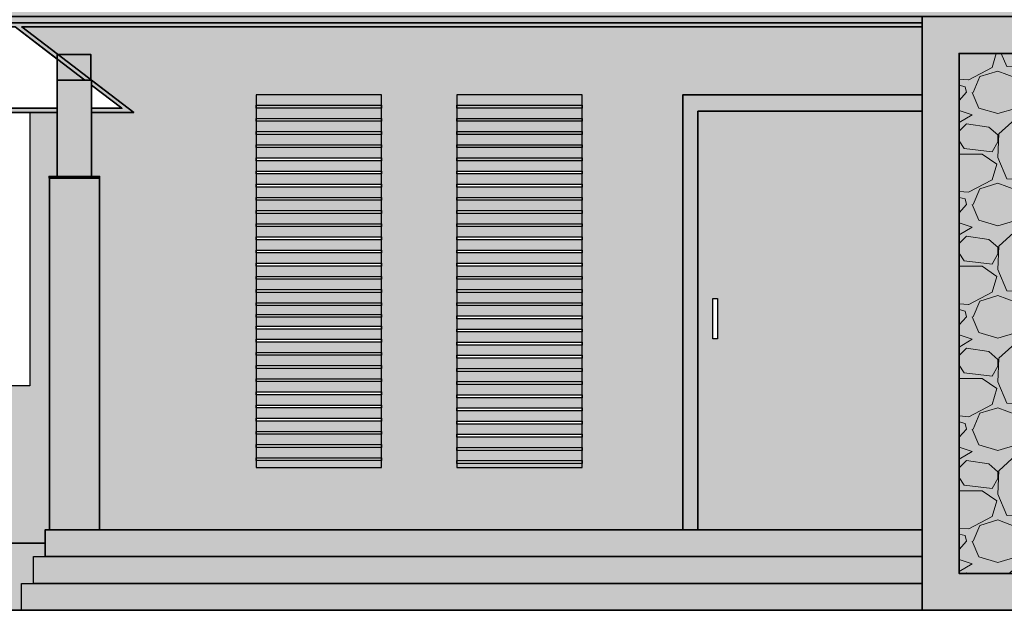
# Model space of a CAD drawing. Units: feet. Extents: x 2613 to 3913, y 950 to 1393.
# Tile 2 of 6: x 2725 to 2948, y 950 to 1083. Entities that reach past the tile are written whole.
import ezdxf

# ---------------------------------------------------------------- set-up
doc = ezdxf.new("R2010")
doc.units = ezdxf.units.FT
for name, color, linetype, lineweight in [('A-DOOR', 3, 'Continuous', 25), ('A-ELEV', 7, 'Continuous', 35), ('A-ELEV-PATT', 9, 'Continuous', 13), ('A-FLOR-STRS', 7, 'Continuous', 25), ('A-GLAZ', 4, 'Continuous', 25)]:
    doc.layers.add(name, color=color, linetype=linetype, lineweight=lineweight)

# ---------------------------------------------------------------- blocks, each defined once
blk = doc.blocks.new('WIN-LOUVRE-SHUTTER-L')
for points in [[(3513.53, 1066.37), (3485.15, 1066.37), (3485.15, 982.04), (3513.53, 982.04)], [(3485.15, 1064.05), (3513.53, 1064.05), (3513.53, 1063.39), (3485.15, 1063.39)], [(3485.15, 1061.07), (3513.53, 1061.07), (3513.53, 1060.41), (3485.15, 1060.41)], [(3485.15, 1058.09), (3513.53, 1058.09), (3513.53, 1057.43), (3485.15, 1057.43)], [(3485.15, 1055.11), (3513.53, 1055.11), (3513.53, 1054.45), (3485.15, 1054.45)], [(3485.15, 1052.13), (3513.53, 1052.13), (3513.53, 1051.47), (3485.15, 1051.47)], [(3485.15, 1049.15), (3513.53, 1049.15), (3513.53, 1048.49), (3485.15, 1048.49)], [(3485.15, 1046.18), (3513.53, 1046.18), (3513.53, 1045.51), (3485.15, 1045.51)], [(3485.15, 1043.2), (3513.53, 1043.2), (3513.53, 1042.53), (3485.15, 1042.53)], [(3485.15, 1040.22), (3513.53, 1040.22), (3513.53, 1039.56), (3485.15, 1039.56)], [(3485.15, 1037.24), (3513.53, 1037.24), (3513.53, 1036.58), (3485.15, 1036.58)], [(3485.15, 1034.26), (3513.53, 1034.26), (3513.53, 1033.6), (3485.15, 1033.6)], [(3485.15, 1031.28), (3513.53, 1031.28), (3513.53, 1030.62), (3485.15, 1030.62)], [(3485.15, 1028.3), (3513.53, 1028.3), (3513.53, 1027.64), (3485.15, 1027.64)], [(3485.15, 1025.32), (3513.53, 1025.32), (3513.53, 1024.66), (3485.15, 1024.66)], [(3485.15, 1022.34), (3513.53, 1022.34), (3513.53, 1021.68), (3485.15, 1021.68)], [(3485.15, 1019.36), (3513.53, 1019.36), (3513.53, 1018.7), (3485.15, 1018.7)], [(3485.15, 1016.71), (3513.53, 1016.71), (3513.53, 1016.05), (3485.15, 1016.05)], [(3485.15, 1014.07), (3513.53, 1014.07), (3513.53, 1013.4), (3485.15, 1013.4)], [(3485.15, 1011.09), (3513.53, 1011.09), (3513.53, 1010.43), (3485.15, 1010.43)], [(3485.15, 1008.11), (3513.53, 1008.11), (3513.53, 1007.45), (3485.15, 1007.45)], [(3485.15, 1005.13), (3513.53, 1005.13), (3513.53, 1004.47), (3485.15, 1004.47)], [(3485.15, 1002.15), (3513.53, 1002.15), (3513.53, 1001.49), (3485.15, 1001.49)], [(3485.15, 999.17), (3513.53, 999.17), (3513.53, 998.51), (3485.15, 998.51)], [(3485.15, 996.19), (3513.53, 996.19), (3513.53, 995.53), (3485.15, 995.53)], [(3485.15, 993.21), (3513.53, 993.21), (3513.53, 992.55), (3485.15, 992.55)], [(3485.15, 990.23), (3513.53, 990.23), (3513.53, 989.57), (3485.15, 989.57)], [(3485.15, 987.25), (3513.53, 987.25), (3513.53, 986.59), (3485.15, 986.59)], [(3485.15, 984.27), (3513.53, 984.27), (3513.53, 983.61), (3485.15, 983.61)]]:
    blk.add_lwpolyline(points, close=True)
blk = doc.blocks.new('WIN-LOUVRE-SHUTTER-R')
for points in [[(3559, 1066.37), (3530.62, 1066.37), (3530.62, 982.04), (3559, 982.04)], [(3530.62, 1064.05), (3559, 1064.05), (3559, 1063.39), (3530.62, 1063.39)], [(3530.62, 1061.07), (3559, 1061.07), (3559, 1060.41), (3530.62, 1060.41)], [(3530.62, 1058.09), (3559, 1058.09), (3559, 1057.43), (3530.62, 1057.43)], [(3530.62, 1055.11), (3559, 1055.11), (3559, 1054.45), (3530.62, 1054.45)], [(3530.62, 1052.13), (3559, 1052.13), (3559, 1051.47), (3530.62, 1051.47)], [(3530.62, 1049.15), (3559, 1049.15), (3559, 1048.49), (3530.62, 1048.49)], [(3530.62, 1046.18), (3559, 1046.18), (3559, 1045.51), (3530.62, 1045.51)], [(3530.62, 1043.2), (3559, 1043.2), (3559, 1042.53), (3530.62, 1042.53)], [(3530.62, 1040.22), (3559, 1040.22), (3559, 1039.56), (3530.62, 1039.56)], [(3530.62, 1037.24), (3559, 1037.24), (3559, 1036.58), (3530.62, 1036.58)], [(3530.62, 1034.26), (3559, 1034.26), (3559, 1033.6), (3530.62, 1033.6)], [(3530.62, 1031.28), (3559, 1031.28), (3559, 1030.62), (3530.62, 1030.62)], [(3530.62, 1028.3), (3559, 1028.3), (3559, 1027.64), (3530.62, 1027.64)], [(3530.62, 1025.32), (3559, 1025.32), (3559, 1024.66), (3530.62, 1024.66)], [(3530.62, 1022.34), (3559, 1022.34), (3559, 1021.68), (3530.62, 1021.68)], [(3530.62, 1019.36), (3559, 1019.36), (3559, 1018.7), (3530.62, 1018.7)], [(3530.62, 1016.38), (3559, 1016.38), (3559, 1015.72), (3530.62, 1015.72)], [(3530.62, 1013.4), (3559, 1013.4), (3559, 1012.74), (3530.62, 1012.74)], [(3530.62, 1010.43), (3559, 1010.43), (3559, 1009.76), (3530.62, 1009.76)], [(3530.62, 1007.45), (3559, 1007.45), (3559, 1006.78), (3530.62, 1006.78)], [(3530.62, 1004.47), (3559, 1004.47), (3559, 1003.81), (3530.62, 1003.81)], [(3530.62, 1001.49), (3559, 1001.49), (3559, 1000.83), (3530.62, 1000.83)], [(3530.62, 998.51), (3559, 998.51), (3559, 997.85), (3530.62, 997.85)], [(3530.62, 995.53), (3559, 995.53), (3559, 994.87), (3530.62, 994.87)], [(3530.62, 992.55), (3559, 992.55), (3559, 991.89), (3530.62, 991.89)], [(3530.62, 989.57), (3559, 989.57), (3559, 988.91), (3530.62, 988.91)], [(3530.62, 986.59), (3559, 986.59), (3559, 985.93), (3530.62, 985.93)], [(3530.62, 983.61), (3559, 983.61), (3559, 982.95), (3530.62, 982.95)]]:
    blk.add_lwpolyline(points, close=True)

msp = doc.modelspace()

# ---------------------------------------------------------------- hatches: boundary and pattern name
at = {"layer": 'A-ELEV-PATT'}
h = msp.add_hatch(color=256, dxfattribs=at)
h.dxf.hatch_style = 1
h.paths.add_polyline_path([(3108.91, 1328.81), (3061.44, 1376.28), (2929.45, 1244.29), (2929.45, 1223.38), (2942.09, 1223.38), (2942.09, 1215.5), (2929.45, 1215.5), (2929.45, 1084.12), (3108.91, 1084.12), (3108.91, 1199.69), (3106.87, 1199.69), (3106.87, 1128.72), (3017.91, 1128.72), (3017.91, 1199.69), (3008.08, 1199.69), (3008.08, 1180.01), (3007.65, 1180.01), (3007.65, 1199.69), (3004.75, 1199.69), (3004.75, 1206.47), (3108.91, 1206.47)])
h.paths.add_polyline_path([(3061.44, 1376.28), (3193.8, 1243.92), (3193.8, 1233.84), (3204.34, 1246.9), (3061.54, 1389.71), (2918.82, 1247), (2929.45, 1233.69), (2929.45, 1244.29)])
h.paths.add_polyline_path([(3061.54, 1389.71), (3204.34, 1246.9), (3206.69, 1248.02), (3061.63, 1393.09), (2916.59, 1248.06), (2918.82, 1247)])
h.paths.add_polyline_path([(2925.65, 1257.12), (2667.59, 1257.12), (2651.33, 1257.12), (2651.33, 1252.28), (2920.82, 1252.28)])
h.paths.add_polyline_path([(2920.82, 1252.28), (2651.33, 1252.28, -0.144454), (2652.15, 1251.12), (2667.59, 1251.12), (2919.65, 1251.12)])
h.paths.add_polyline_path([(2918.82, 1247), (2916.59, 1248.06), (2919.65, 1251.12), (2667.59, 1251.12), (2652.15, 1251.12), (2667.59, 1229.14), (2667.59, 1233.69), (2929.45, 1233.69)])
h.paths.add_polyline_path([(2710.6, 1223.38), (2929.45, 1223.38), (2929.45, 1233.69), (2667.59, 1233.69), (2667.59, 1229.14), (2667.59, 1201.16), (2720.67, 1201.16), (2710.6, 1215.5)])
h.paths.add_polyline_path([(2942.09, 1223.38), (2710.6, 1223.38), (2710.6, 1215.5), (2921.48, 1215.5), (2942.09, 1215.5)])
h.paths.add_polyline_path([(2929.45, 1215.5), (2921.48, 1215.5), (2710.6, 1215.5), (2733.47, 1182.94), (2733.47, 1195.74), (2741.22, 1195.74), (2929.45, 1195.74)])
h.paths.add_polyline_path([(2721, 1200.68), (2661.89, 1200.68), (2661.89, 1195.74), (2724.47, 1195.74)])
h.paths.add_polyline_path([(2733.47, 1182.94), (2727.27, 1191.76), (2727.27, 1133.88), (2731.7, 1133.88), (2731.7, 1169.74), (2731.61, 1169.74), (2731.61, 1170.13), (2733.47, 1170.13)])
h.paths.add_polyline_path([(2929.45, 1183.04), (2741.22, 1183.04), (2741.22, 1170.13), (2743.07, 1170.13), (2743.07, 1169.74), (2743.07, 1112.32), (2759.57, 1112.32), (2759.57, 1167.82), (2763.7, 1167.82), (2763.7, 1112.32), (2781.75, 1112.32), (2781.75, 1167.82), (2785.87, 1167.82), (2785.87, 1112.32), (2803.92, 1112.32), (2803.92, 1167.82), (2808.05, 1167.82), (2808.05, 1112.32), (2826.09, 1112.32), (2826.09, 1167.82), (2830.22, 1167.82), (2830.22, 1112.32), (2875.17, 1112.32), (2875.17, 1171.49), (2929.45, 1171.49)])
h.paths.add_polyline_path([(2731.7, 1133.88), (2661.89, 1133.88), (2661.89, 1084.12), (2730.99, 1084.12), (2730.99, 1112.32), (2731.7, 1112.32)])
h.paths.add_polyline_path([(2929.45, 1112.32), (2730.99, 1112.32), (2730.99, 1084.12), (2929.45, 1084.12)])
h.paths.add_polyline_path([(2929.45, 1084.12), (2730.99, 1084.12), (2661.89, 1084.12), (2612.72, 1084.12), (2612.72, 1082.68), (2929.45, 1082.68)])
h.paths.add_polyline_path([(2929.45, 1082.68), (2612.72, 1082.68), (2639.32, 1062.44), (2733.47, 1062.44), (2733.47, 1063.35), (2639.62, 1063.35), (2615.43, 1081.77), (2723.91, 1081.77), (2739.71, 1069.74), (2741.22, 1069.74), (2725.42, 1081.77), (2929.45, 1081.77)])
h.paths.add_polyline_path([(2671.42, 1081.77), (2668.07, 1081.77), (2692.27, 1063.35), (2695.62, 1063.35)], flags=17)
h.paths.add_polyline_path([(2741.22, 1069.74), (2741.22, 1068.59), (2748.11, 1063.35), (2741.22, 1063.35), (2741.22, 1062.44), (2750.82, 1062.44)], flags=17)
h.paths.add_polyline_path([(2929.45, 1081.77), (2725.42, 1081.77), (2750.82, 1062.44), (2741.22, 1062.44), (2741.22, 1047.95), (2743.07, 1047.95), (2743.07, 1047.56), (2743.07, 967.97), (2875.17, 967.97), (2875.17, 1066.37), (2929.45, 1066.37)])
h.paths.add_polyline_path([(2778.55, 1066.37), (2806.94, 1066.37), (2806.94, 982.04), (2778.55, 982.04)], flags=16)
h.paths.add_polyline_path([(2778.55, 1064.05), (2806.94, 1064.05), (2806.94, 1063.39), (2778.55, 1063.39)], flags=16)
h.paths.add_polyline_path([(2778.55, 1061.07), (2806.94, 1061.07), (2806.94, 1060.41), (2778.55, 1060.41)], flags=0)
h.paths.add_polyline_path([(2778.55, 1058.09), (2806.94, 1058.09), (2806.94, 1057.43), (2778.55, 1057.43)], flags=0)
h.paths.add_polyline_path([(2778.55, 1055.11), (2806.94, 1055.11), (2806.94, 1054.45), (2778.55, 1054.45)], flags=0)
h.paths.add_polyline_path([(2778.55, 1052.13), (2806.94, 1052.13), (2806.94, 1051.47), (2778.55, 1051.47)], flags=0)
h.paths.add_polyline_path([(2778.55, 1049.15), (2806.94, 1049.15), (2806.94, 1048.49), (2778.55, 1048.49)], flags=0)
h.paths.add_polyline_path([(2778.55, 1046.18), (2806.94, 1046.18), (2806.94, 1045.51), (2778.55, 1045.51)], flags=0)
h.paths.add_polyline_path([(2778.55, 1043.2), (2806.94, 1043.2), (2806.94, 1042.53), (2778.55, 1042.53)], flags=0)
h.paths.add_polyline_path([(2778.55, 1040.22), (2806.94, 1040.22), (2806.94, 1039.56), (2778.55, 1039.56)], flags=0)
h.paths.add_polyline_path([(2778.55, 1037.24), (2806.94, 1037.24), (2806.94, 1036.58), (2778.55, 1036.58)], flags=0)
h.paths.add_polyline_path([(2778.55, 1034.26), (2806.94, 1034.26), (2806.94, 1033.6), (2778.55, 1033.6)], flags=0)
h.paths.add_polyline_path([(2778.55, 1031.28), (2806.94, 1031.28), (2806.94, 1030.62), (2778.55, 1030.62)], flags=0)
h.paths.add_polyline_path([(2778.55, 1028.3), (2806.94, 1028.3), (2806.94, 1027.64), (2778.55, 1027.64)], flags=0)
h.paths.add_polyline_path([(2778.55, 1025.32), (2806.94, 1025.32), (2806.94, 1024.66), (2778.55, 1024.66)], flags=0)
h.paths.add_polyline_path([(2778.55, 1022.34), (2806.94, 1022.34), (2806.94, 1021.68), (2778.55, 1021.68)], flags=0)
h.paths.add_polyline_path([(2778.55, 1019.36), (2806.94, 1019.36), (2806.94, 1018.7), (2778.55, 1018.7)], flags=0)
h.paths.add_polyline_path([(2778.55, 1016.71), (2806.94, 1016.71), (2806.94, 1016.05), (2778.55, 1016.05)], flags=0)
h.paths.add_polyline_path([(2824.02, 1066.37), (2852.41, 1066.37), (2852.41, 982.04), (2824.02, 982.04)], flags=16)
h.paths.add_polyline_path([(2778.55, 1014.07), (2806.94, 1014.07), (2806.94, 1013.4), (2778.55, 1013.4)], flags=0)
h.paths.add_polyline_path([(2824.02, 1064.05), (2852.41, 1064.05), (2852.41, 1063.39), (2824.02, 1063.39)], flags=16)
h.paths.add_polyline_path([(2824.02, 1061.07), (2852.41, 1061.07), (2852.41, 1060.41), (2824.02, 1060.41)], flags=0)
h.paths.add_polyline_path([(2824.02, 1058.09), (2852.41, 1058.09), (2852.41, 1057.43), (2824.02, 1057.43)], flags=0)
h.paths.add_polyline_path([(2824.02, 1055.11), (2852.41, 1055.11), (2852.41, 1054.45), (2824.02, 1054.45)], flags=16)
h.paths.add_polyline_path([(2824.02, 1052.13), (2852.41, 1052.13), (2852.41, 1051.47), (2824.02, 1051.47)], flags=0)
h.paths.add_polyline_path([(2778.55, 1011.09), (2806.94, 1011.09), (2806.94, 1010.43), (2778.55, 1010.43)], flags=0)
h.paths.add_polyline_path([(2824.02, 1049.15), (2852.41, 1049.15), (2852.41, 1048.49), (2824.02, 1048.49)], flags=0)
h.paths.add_polyline_path([(2824.02, 1046.18), (2852.41, 1046.18), (2852.41, 1045.51), (2824.02, 1045.51)], flags=0)
h.paths.add_polyline_path([(2824.02, 1043.2), (2852.41, 1043.2), (2852.41, 1042.53), (2824.02, 1042.53)], flags=0)
h.paths.add_polyline_path([(2778.55, 1008.11), (2806.94, 1008.11), (2806.94, 1007.45), (2778.55, 1007.45)], flags=0)
h.paths.add_polyline_path([(2824.02, 1040.22), (2852.41, 1040.22), (2852.41, 1039.56), (2824.02, 1039.56)], flags=0)
h.paths.add_polyline_path([(2824.02, 1037.24), (2852.41, 1037.24), (2852.41, 1036.58), (2824.02, 1036.58)], flags=0)
h.paths.add_polyline_path([(2778.55, 1005.13), (2806.94, 1005.13), (2806.94, 1004.47), (2778.55, 1004.47)], flags=0)
h.paths.add_polyline_path([(2824.02, 1034.26), (2852.41, 1034.26), (2852.41, 1033.6), (2824.02, 1033.6)], flags=0)
h.paths.add_polyline_path([(2824.02, 1031.28), (2852.41, 1031.28), (2852.41, 1030.62), (2824.02, 1030.62)], flags=0)
h.paths.add_polyline_path([(2778.55, 1002.15), (2806.94, 1002.15), (2806.94, 1001.49), (2778.55, 1001.49)], flags=0)
h.paths.add_polyline_path([(2824.02, 1028.3), (2852.41, 1028.3), (2852.41, 1027.64), (2824.02, 1027.64)], flags=0)
h.paths.add_polyline_path([(2778.55, 999.17), (2806.94, 999.17), (2806.94, 998.51), (2778.55, 998.51)], flags=0)
h.paths.add_polyline_path([(2824.02, 1025.32), (2852.41, 1025.32), (2852.41, 1024.66), (2824.02, 1024.66)], flags=0)
h.paths.add_polyline_path([(2824.02, 1022.34), (2852.41, 1022.34), (2852.41, 1021.68), (2824.02, 1021.68)], flags=0)
h.paths.add_polyline_path([(2778.55, 996.19), (2806.94, 996.19), (2806.94, 995.53), (2778.55, 995.53)], flags=0)
h.paths.add_polyline_path([(2824.02, 1019.36), (2852.41, 1019.36), (2852.41, 1018.7), (2824.02, 1018.7)], flags=0)
h.paths.add_polyline_path([(2778.55, 993.21), (2806.94, 993.21), (2806.94, 992.55), (2778.55, 992.55)], flags=0)
h.paths.add_polyline_path([(2824.02, 1016.38), (2852.41, 1016.38), (2852.41, 1015.72), (2824.02, 1015.72)], flags=0)
h.paths.add_polyline_path([(2824.02, 1013.4), (2852.41, 1013.4), (2852.41, 1012.74), (2824.02, 1012.74)], flags=0)
h.paths.add_polyline_path([(2778.55, 990.23), (2806.94, 990.23), (2806.94, 989.57), (2778.55, 989.57)], flags=0)
h.paths.add_polyline_path([(2824.02, 1010.43), (2852.41, 1010.43), (2852.41, 1009.76), (2824.02, 1009.76)], flags=0)
h.paths.add_polyline_path([(2778.55, 987.25), (2806.94, 987.25), (2806.94, 986.59), (2778.55, 986.59)], flags=0)
h.paths.add_polyline_path([(2824.02, 1007.45), (2852.41, 1007.45), (2852.41, 1006.78), (2824.02, 1006.78)], flags=0)
h.paths.add_polyline_path([(2778.55, 984.27), (2806.94, 984.27), (2806.94, 983.61), (2778.55, 983.61)], flags=0)
h.paths.add_polyline_path([(2824.02, 1004.47), (2852.41, 1004.47), (2852.41, 1003.81), (2824.02, 1003.81)], flags=0)
h.paths.add_polyline_path([(2824.02, 1001.49), (2852.41, 1001.49), (2852.41, 1000.83), (2824.02, 1000.83)], flags=0)
h.paths.add_polyline_path([(2824.02, 998.51), (2852.41, 998.51), (2852.41, 997.85), (2824.02, 997.85)], flags=0)
h.paths.add_polyline_path([(2824.02, 995.53), (2852.41, 995.53), (2852.41, 994.87), (2824.02, 994.87)], flags=0)
h.paths.add_polyline_path([(2824.02, 992.55), (2852.41, 992.55), (2852.41, 991.89), (2824.02, 991.89)], flags=0)
h.paths.add_polyline_path([(2824.02, 989.57), (2852.41, 989.57), (2852.41, 988.91), (2824.02, 988.91)], flags=0)
h.paths.add_polyline_path([(2824.02, 986.59), (2852.41, 986.59), (2852.41, 985.93), (2824.02, 985.93)], flags=0)
h.paths.add_polyline_path([(2824.02, 983.61), (2852.41, 983.61), (2852.41, 982.95), (2824.02, 982.95)], flags=0)
h.paths.add_polyline_path([(2731.7, 1047.56), (2731.61, 1047.56), (2731.61, 1047.95), (2733.47, 1047.95), (2733.47, 1062.44), (2727.27, 1062.44), (2727.27, 1000.58), (2667.59, 1000.58), (2667.59, 1062.44), (2664.87, 1062.44), (2664.87, 965.01), (2730.76, 964.93), (2730.76, 967.97), (2731.7, 967.97)])
h.paths.add_polyline_path([(2728.06, 961.9), (2730.76, 961.9), (2730.76, 964.93), (2663.94, 964.93), (2663.94, 949.74), (2725.36, 949.74), (2725.36, 955.82), (2728.06, 955.82)])
h.paths.add_polyline_path([(2929.45, 967.97), (2730.76, 967.97), (2730.76, 961.9), (2929.45, 961.9)])
h.paths.add_polyline_path([(2929.45, 961.9), (2730.76, 961.9), (2728.06, 961.9), (2728.06, 955.82), (2929.45, 955.82)])
h.paths.add_polyline_path([(2929.45, 955.82), (2728.06, 955.82), (2725.36, 955.82), (2725.36, 949.74), (2929.45, 949.74)])
h.paths.add_polyline_path([(2741.22, 1069.74), (2733.47, 1069.74), (2733.47, 1047.95), (2741.22, 1047.95)], flags=17)
h.paths.add_polyline_path([(2741.22, 1195.74), (2733.47, 1195.74), (2733.47, 1182.94), (2733.47, 1170.13), (2741.22, 1170.13), (2741.22, 1183.04)])
h.paths.add_polyline_path([(3193.8, 1084.12), (2929.45, 1084.12), (2929.45, 1082.68), (2929.45, 1081.77), (2929.45, 1066.37), (2929.45, 949.74), (3193.8, 949.74)])
h.paths.add_polyline_path([(2937.79, 1075.78), (3185.46, 1075.78), (3185.46, 958.09), (2937.79, 958.09)], flags=16)
h.paths.add_polyline_path([(3011.76, 1075.78), (3104.46, 1075.78), (3104.46, 993.6), (3011.76, 993.6)], flags=0)
h.paths.add_polyline_path([(3015.24, 1075.78), (3016.57, 1075.78), (3016.57, 1060.85), (3043.1, 1060.85), (3043.1, 1075.78), (3045.77, 1075.78), (3045.77, 997.08), (3070.45, 997.08), (3070.45, 1075.78), (3073.12, 1075.78), (3073.12, 1060.85), (3099.64, 1060.85), (3099.64, 1075.78), (3100.98, 1075.78), (3100.98, 997.08), (3099.64, 997.08), (3015.24, 997.08)], flags=0)
h = msp.add_hatch(color=256, dxfattribs=at)
h.dxf.hatch_style = 1
h.paths.add_polyline_path([(2768.1, 1195.09), (2741.95, 1195.09), (2741.95, 1183.7), (2768.1, 1183.7)])
h.paths.add_polyline_path([(2794.91, 1195.09), (2768.76, 1195.09), (2768.76, 1183.7), (2794.91, 1183.7)])
h.paths.add_polyline_path([(2821.72, 1195.09), (2795.57, 1195.09), (2795.57, 1183.7), (2821.72, 1183.7)])
h.paths.add_polyline_path([(2848.53, 1195.09), (2822.38, 1195.09), (2822.38, 1183.7), (2848.53, 1183.7)])
h.paths.add_polyline_path([(2875.34, 1195.09), (2849.19, 1195.09), (2849.19, 1183.7), (2875.34, 1183.7)])
h.paths.add_polyline_path([(2683.29, 1193.04), (2670.29, 1193.04), (2670.29, 1190.17), (2683.29, 1190.17)])
h.paths.add_polyline_path([(2696.31, 1193.04), (2683.32, 1193.04), (2683.32, 1190.17), (2696.31, 1190.17)])
h.paths.add_polyline_path([(2696.31, 1190.14), (2683.32, 1190.14), (2683.32, 1187.27), (2696.31, 1187.27)])
h.paths.add_polyline_path([(2683.29, 1190.14), (2670.29, 1190.14), (2670.29, 1187.27), (2683.29, 1187.27)])
h.paths.add_polyline_path([(2683.29, 1187.24), (2670.29, 1187.24), (2670.29, 1184.37), (2683.29, 1184.37)])
h.paths.add_polyline_path([(2696.31, 1187.24), (2683.32, 1187.24), (2683.32, 1184.37), (2696.31, 1184.37)])
h.paths.add_polyline_path([(2683.29, 1184.34), (2670.29, 1184.34), (2670.29, 1181.47), (2683.29, 1181.47)])
h.paths.add_polyline_path([(2696.31, 1184.34), (2683.32, 1184.34), (2683.32, 1181.47), (2696.31, 1181.47)])
h.paths.add_polyline_path([(2683.29, 1181.44), (2670.29, 1181.44), (2670.29, 1178.57), (2683.29, 1178.57)])
h.paths.add_polyline_path([(2696.31, 1181.44), (2683.32, 1181.44), (2683.32, 1178.57), (2696.31, 1178.57)])
h.paths.add_polyline_path([(2696.31, 1178.53), (2683.32, 1178.53), (2683.32, 1175.67), (2696.31, 1175.67)])
h.paths.add_polyline_path([(2683.29, 1178.53), (2670.29, 1178.53), (2670.29, 1175.67), (2683.29, 1175.67)])
h.paths.add_polyline_path([(2683.29, 1175.63), (2670.29, 1175.63), (2670.29, 1172.76), (2683.29, 1172.76)])
h.paths.add_polyline_path([(2696.31, 1175.63), (2683.32, 1175.63), (2683.32, 1172.76), (2696.31, 1172.76)])
h.paths.add_polyline_path([(2683.29, 1172.73), (2670.29, 1172.73), (2670.29, 1169.86), (2683.29, 1169.86)])
h.paths.add_polyline_path([(2696.31, 1172.73), (2683.32, 1172.73), (2683.32, 1169.86), (2696.31, 1169.86)])
h.paths.add_polyline_path([(2696.31, 1169.83), (2683.32, 1169.83), (2683.32, 1166.96), (2696.31, 1166.96)])
h.paths.add_polyline_path([(2683.29, 1169.83), (2670.29, 1169.83), (2670.29, 1166.96), (2683.29, 1166.96)])
h.paths.add_polyline_path([(2696.31, 1166.93), (2683.32, 1166.93), (2683.32, 1164.06), (2696.31, 1164.06)])
h.paths.add_polyline_path([(2683.29, 1166.93), (2670.29, 1166.93), (2670.29, 1164.06), (2683.29, 1164.06)])
h.paths.add_polyline_path([(2683.29, 1164.03), (2670.29, 1164.03), (2670.29, 1161.16), (2683.29, 1161.16)])
h.paths.add_polyline_path([(2696.31, 1164.03), (2683.32, 1164.03), (2683.32, 1161.16), (2696.31, 1161.16)])
h.paths.add_polyline_path([(2696.31, 1161.12), (2683.32, 1161.12), (2683.32, 1158.25), (2696.31, 1158.25)])
h.paths.add_polyline_path([(2683.29, 1161.12), (2670.29, 1161.12), (2670.29, 1158.25), (2683.29, 1158.25)])
h.paths.add_polyline_path([(2683.29, 1158.22), (2670.29, 1158.22), (2670.29, 1155.35), (2683.29, 1155.35)])
h.paths.add_polyline_path([(2696.31, 1158.22), (2683.32, 1158.22), (2683.32, 1155.35), (2696.31, 1155.35)])
h.paths.add_polyline_path([(2696.31, 1155.32), (2683.32, 1155.32), (2683.32, 1152.45), (2696.31, 1152.45)])
h.paths.add_polyline_path([(2683.29, 1155.32), (2670.29, 1155.32), (2670.29, 1152.45), (2683.29, 1152.45)])
h.paths.add_polyline_path([(2683.29, 1152.42), (2670.29, 1152.42), (2670.29, 1149.55), (2683.29, 1149.55)])
h.paths.add_polyline_path([(2696.31, 1152.42), (2683.32, 1152.42), (2683.32, 1149.55), (2696.31, 1149.55)])
h.paths.add_polyline_path([(2683.29, 1149.52), (2670.29, 1149.52), (2670.29, 1146.65), (2683.29, 1146.65)])
h.paths.add_polyline_path([(2696.31, 1149.52), (2683.32, 1149.52), (2683.32, 1146.65), (2696.31, 1146.65)])
h.paths.add_polyline_path([(2696.31, 1146.61), (2683.32, 1146.61), (2683.32, 1143.75), (2696.31, 1143.75)])
h.paths.add_polyline_path([(2683.29, 1146.61), (2670.29, 1146.61), (2670.29, 1143.75), (2683.29, 1143.75)])
h.paths.add_polyline_path([(2683.29, 1143.71), (2670.29, 1143.71), (2670.29, 1140.84), (2683.29, 1140.84)])
h.paths.add_polyline_path([(2696.31, 1143.71), (2683.32, 1143.71), (2683.32, 1140.84), (2696.31, 1140.84)])
h.paths.add_polyline_path([(2683.29, 1140.81), (2670.29, 1140.81), (2670.29, 1137.94), (2683.29, 1137.94)])
h.paths.add_polyline_path([(2696.31, 1140.81), (2683.32, 1140.81), (2683.32, 1137.94), (2696.31, 1137.94)])
h.paths.add_polyline_path([(2683.29, 1137.91), (2670.29, 1137.91), (2670.29, 1136.58), (2683.29, 1136.58)])
h.paths.add_polyline_path([(2696.31, 1137.91), (2683.32, 1137.91), (2683.32, 1136.58), (2696.31, 1136.58)])
h.paths.add_polyline_path([(3074.7, 1198.4), (3050.02, 1198.4), (3050.02, 1130.01), (3074.7, 1130.01)])
h.paths.add_polyline_path([(3047.34, 1198.4), (3019.29, 1198.4), (3019.29, 1184.76), (3047.34, 1184.76)])
h.paths.add_polyline_path([(3047.34, 1183.78), (3019.29, 1183.78), (3019.29, 1130.01), (3047.34, 1130.01)])
h.paths.add_polyline_path([(3105.48, 1198.4), (3077.37, 1198.4), (3077.37, 1184.76), (3105.48, 1184.76)])
h.paths.add_polyline_path([(3105.48, 1183.78), (3077.37, 1183.78), (3077.37, 1130.01), (3105.48, 1130.01)])
h.paths.add_polyline_path([(3070.45, 1075.78), (3045.77, 1075.78), (3045.77, 997.08), (3070.45, 997.08)])
h.paths.add_polyline_path([(3099.64, 1075.78), (3073.12, 1075.78), (3073.12, 1060.85), (3099.64, 1060.85)])
h.paths.add_polyline_path([(3099.64, 1059.87), (3073.12, 1059.87), (3073.12, 997.08), (3099.64, 997.08)])
h.paths.add_polyline_path([(3043.1, 1075.78), (3016.57, 1075.78), (3016.57, 1060.85), (3043.1, 1060.85)])
h.paths.add_polyline_path([(3043.1, 1059.87), (3016.57, 1059.87), (3016.57, 997.08), (3043.1, 997.08)])
h.paths.add_polyline_path([(2683.29, 1059.73), (2670.29, 1059.73), (2670.29, 1056.87), (2683.29, 1056.87)])
h.paths.add_polyline_path([(2696.31, 1059.73), (2683.32, 1059.73), (2683.32, 1056.87), (2696.31, 1056.87)])
h.paths.add_polyline_path([(2696.31, 1056.83), (2683.32, 1056.83), (2683.32, 1053.96), (2696.31, 1053.96)])
h.paths.add_polyline_path([(2683.29, 1056.83), (2670.29, 1056.83), (2670.29, 1053.96), (2683.29, 1053.96)])
h.paths.add_polyline_path([(2683.29, 1053.93), (2670.29, 1053.93), (2670.29, 1051.06), (2683.29, 1051.06)])
h.paths.add_polyline_path([(2696.31, 1053.93), (2683.32, 1053.93), (2683.32, 1051.06), (2696.31, 1051.06)])
h.paths.add_polyline_path([(2683.29, 1051.03), (2670.29, 1051.03), (2670.29, 1048.16), (2683.29, 1048.16)])
h.paths.add_polyline_path([(2696.31, 1051.03), (2683.32, 1051.03), (2683.32, 1048.16), (2696.31, 1048.16)])
h.paths.add_polyline_path([(2683.29, 1048.13), (2670.29, 1048.13), (2670.29, 1045.26), (2683.29, 1045.26)])
h.paths.add_polyline_path([(2696.31, 1048.13), (2683.32, 1048.13), (2683.32, 1045.26), (2696.31, 1045.26)])
h.paths.add_polyline_path([(2696.31, 1045.23), (2683.32, 1045.23), (2683.32, 1042.36), (2696.31, 1042.36)])
h.paths.add_polyline_path([(2683.29, 1045.23), (2670.29, 1045.23), (2670.29, 1042.36), (2683.29, 1042.36)])
h.paths.add_polyline_path([(2683.29, 1042.32), (2670.29, 1042.32), (2670.29, 1039.46), (2683.29, 1039.46)])
h.paths.add_polyline_path([(2696.31, 1042.32), (2683.32, 1042.32), (2683.32, 1039.46), (2696.31, 1039.46)])
h.paths.add_polyline_path([(2696.31, 1039.42), (2683.32, 1039.42), (2683.32, 1036.55), (2696.31, 1036.55)])
h.paths.add_polyline_path([(2683.29, 1039.42), (2670.29, 1039.42), (2670.29, 1036.55), (2683.29, 1036.55)])
h.paths.add_polyline_path([(2683.29, 1036.52), (2670.29, 1036.52), (2670.29, 1033.65), (2683.29, 1033.65)])
h.paths.add_polyline_path([(2696.31, 1036.52), (2683.32, 1036.52), (2683.32, 1033.65), (2696.31, 1033.65)])
h.paths.add_polyline_path([(2696.31, 1033.62), (2683.32, 1033.62), (2683.32, 1030.75), (2696.31, 1030.75)])
h.paths.add_polyline_path([(2683.29, 1033.62), (2670.29, 1033.62), (2670.29, 1030.75), (2683.29, 1030.75)])
h.paths.add_polyline_path([(2696.31, 1030.72), (2683.32, 1030.72), (2683.32, 1027.85), (2696.31, 1027.85)])
h.paths.add_polyline_path([(2683.29, 1030.72), (2670.29, 1030.72), (2670.29, 1027.85), (2683.29, 1027.85)])
h.paths.add_polyline_path([(2683.29, 1027.82), (2670.29, 1027.82), (2670.29, 1024.95), (2683.29, 1024.95)])
h.paths.add_polyline_path([(2696.31, 1027.82), (2683.32, 1027.82), (2683.32, 1024.95), (2696.31, 1024.95)])
h.paths.add_polyline_path([(2696.31, 1024.91), (2683.32, 1024.91), (2683.32, 1022.05), (2696.31, 1022.05)])
h.paths.add_polyline_path([(2683.29, 1024.91), (2670.29, 1024.91), (2670.29, 1022.05), (2683.29, 1022.05)])
h.paths.add_polyline_path([(2683.29, 1022.01), (2670.29, 1022.01), (2670.29, 1019.14), (2683.29, 1019.14)])
h.paths.add_polyline_path([(2696.31, 1022.01), (2683.32, 1022.01), (2683.32, 1019.14), (2696.31, 1019.14)])
h.paths.add_polyline_path([(2696.31, 1019.11), (2683.32, 1019.11), (2683.32, 1016.24), (2696.31, 1016.24)])
h.paths.add_polyline_path([(2683.29, 1019.11), (2670.29, 1019.11), (2670.29, 1016.24), (2683.29, 1016.24)])
h.paths.add_polyline_path([(2683.29, 1016.21), (2670.29, 1016.21), (2670.29, 1013.34), (2683.29, 1013.34)])
h.paths.add_polyline_path([(2696.31, 1016.21), (2683.32, 1016.21), (2683.32, 1013.34), (2696.31, 1013.34)])
h.paths.add_polyline_path([(2696.31, 1013.31), (2683.32, 1013.31), (2683.32, 1010.44), (2696.31, 1010.44)])
h.paths.add_polyline_path([(2683.29, 1013.31), (2670.29, 1013.31), (2670.29, 1010.44), (2683.29, 1010.44)])
h.paths.add_polyline_path([(2683.29, 1010.41), (2670.29, 1010.41), (2670.29, 1007.54), (2683.29, 1007.54)])
h.paths.add_polyline_path([(2696.31, 1010.41), (2683.32, 1010.41), (2683.32, 1007.54), (2696.31, 1007.54)])
h.paths.add_polyline_path([(2696.31, 1007.5), (2683.32, 1007.5), (2683.32, 1004.64), (2696.31, 1004.64)])
h.paths.add_polyline_path([(2683.29, 1007.5), (2670.29, 1007.5), (2670.29, 1004.64), (2683.29, 1004.64)])
h.paths.add_polyline_path([(2683.29, 1004.6), (2670.29, 1004.6), (2670.29, 1003.28), (2683.29, 1003.28)])
h.paths.add_polyline_path([(2696.31, 1004.6), (2683.32, 1004.6), (2683.32, 1003.28), (2696.31, 1003.28)])
h.paths.add_polyline_path([(2806.94, 1066.37), (2778.55, 1066.37), (2778.55, 1064.05), (2806.94, 1064.05)])
h.paths.add_polyline_path([(2806.94, 1063.39), (2778.55, 1063.39), (2778.55, 1061.07), (2806.94, 1061.07)])
h.paths.add_polyline_path([(2806.94, 1060.41), (2778.55, 1060.41), (2778.55, 1058.09), (2806.94, 1058.09)])
h.paths.add_polyline_path([(2806.94, 1057.43), (2778.55, 1057.43), (2778.55, 1055.11), (2806.94, 1055.11)])
h.paths.add_polyline_path([(2806.94, 1054.45), (2778.55, 1054.45), (2778.55, 1052.13), (2806.94, 1052.13)])
h.paths.add_polyline_path([(2806.94, 1051.47), (2778.55, 1051.47), (2778.55, 1049.15), (2806.94, 1049.15)])
h.paths.add_polyline_path([(2806.94, 1048.49), (2778.55, 1048.49), (2778.55, 1046.18), (2806.94, 1046.18)])
h.paths.add_polyline_path([(2806.94, 1045.51), (2778.55, 1045.51), (2778.55, 1043.2), (2806.94, 1043.2)])
h.paths.add_polyline_path([(2806.94, 1042.53), (2778.55, 1042.53), (2778.55, 1040.22), (2806.94, 1040.22)])
h.paths.add_polyline_path([(2806.94, 1039.56), (2778.55, 1039.56), (2778.55, 1037.24), (2806.94, 1037.24)])
h.paths.add_polyline_path([(2806.94, 1036.58), (2778.55, 1036.58), (2778.55, 1034.26), (2806.94, 1034.26)])
h.paths.add_polyline_path([(2806.94, 1033.6), (2778.55, 1033.6), (2778.55, 1031.28), (2806.94, 1031.28)])
h.paths.add_polyline_path([(2806.94, 1030.62), (2778.55, 1030.62), (2778.55, 1028.3), (2806.94, 1028.3)])
h.paths.add_polyline_path([(2806.94, 1027.64), (2778.55, 1027.64), (2778.55, 1025.32), (2806.94, 1025.32)])
h.paths.add_polyline_path([(2806.94, 1024.66), (2778.55, 1024.66), (2778.55, 1022.34), (2806.94, 1022.34)])
h.paths.add_polyline_path([(2806.94, 1021.68), (2778.55, 1021.68), (2778.55, 1019.36), (2806.94, 1019.36)])
h.paths.add_polyline_path([(2806.94, 1018.7), (2778.55, 1018.7), (2778.55, 1016.71), (2806.94, 1016.71)])
h.paths.add_polyline_path([(2806.94, 1016.05), (2778.55, 1016.05), (2778.55, 1014.07), (2806.94, 1014.07)])
h.paths.add_polyline_path([(2806.94, 1013.4), (2778.55, 1013.4), (2778.55, 1011.09), (2806.94, 1011.09)])
h.paths.add_polyline_path([(2806.94, 1010.43), (2778.55, 1010.43), (2778.55, 1008.11), (2806.94, 1008.11)])
h.paths.add_polyline_path([(2806.94, 1007.45), (2778.55, 1007.45), (2778.55, 1005.13), (2806.94, 1005.13)])
h.paths.add_polyline_path([(2806.94, 1004.47), (2778.55, 1004.47), (2778.55, 1002.15), (2806.94, 1002.15)])
h.paths.add_polyline_path([(2806.94, 1001.49), (2778.55, 1001.49), (2778.55, 999.17), (2806.94, 999.17)])
h.paths.add_polyline_path([(2806.94, 998.51), (2778.55, 998.51), (2778.55, 996.19), (2806.94, 996.19)])
h.paths.add_polyline_path([(2806.94, 983.61), (2778.55, 983.61), (2778.55, 982.04), (2806.94, 982.04)])
h.paths.add_polyline_path([(2806.94, 986.59), (2778.55, 986.59), (2778.55, 984.27), (2806.94, 984.27)])
h.paths.add_polyline_path([(2806.94, 989.57), (2778.55, 989.57), (2778.55, 987.25), (2806.94, 987.25)])
h.paths.add_polyline_path([(2806.94, 992.55), (2778.55, 992.55), (2778.55, 990.23), (2806.94, 990.23)])
h.paths.add_polyline_path([(2806.94, 995.53), (2778.55, 995.53), (2778.55, 993.21), (2806.94, 993.21)])
h.paths.add_polyline_path([(2852.41, 985.93), (2824.02, 985.93), (2824.02, 983.61), (2852.41, 983.61)])
h.paths.add_polyline_path([(2852.41, 982.95), (2824.02, 982.95), (2824.02, 982.04), (2852.41, 982.04)])
h.paths.add_polyline_path([(2852.41, 988.91), (2824.02, 988.91), (2824.02, 986.59), (2852.41, 986.59)])
h.paths.add_polyline_path([(2852.41, 991.89), (2824.02, 991.89), (2824.02, 989.57), (2852.41, 989.57)])
h.paths.add_polyline_path([(2852.41, 994.87), (2824.02, 994.87), (2824.02, 992.55), (2852.41, 992.55)])
h.paths.add_polyline_path([(2852.41, 997.85), (2824.02, 997.85), (2824.02, 995.53), (2852.41, 995.53)])
h.paths.add_polyline_path([(2852.41, 1000.83), (2824.02, 1000.83), (2824.02, 998.51), (2852.41, 998.51)])
h.paths.add_polyline_path([(2852.41, 1003.81), (2824.02, 1003.81), (2824.02, 1001.49), (2852.41, 1001.49)])
h.paths.add_polyline_path([(2852.41, 1006.78), (2824.02, 1006.78), (2824.02, 1004.47), (2852.41, 1004.47)])
h.paths.add_polyline_path([(2852.41, 1009.76), (2824.02, 1009.76), (2824.02, 1007.45), (2852.41, 1007.45)])
h.paths.add_polyline_path([(2852.41, 1012.74), (2824.02, 1012.74), (2824.02, 1010.43), (2852.41, 1010.43)])
h.paths.add_polyline_path([(2852.41, 1015.72), (2824.02, 1015.72), (2824.02, 1013.4), (2852.41, 1013.4)])
h.paths.add_polyline_path([(2852.41, 1018.7), (2824.02, 1018.7), (2824.02, 1016.38), (2852.41, 1016.38)])
h.paths.add_polyline_path([(2852.41, 1021.68), (2824.02, 1021.68), (2824.02, 1019.36), (2852.41, 1019.36)])
h.paths.add_polyline_path([(2852.41, 1024.66), (2824.02, 1024.66), (2824.02, 1022.34), (2852.41, 1022.34)])
h.paths.add_polyline_path([(2852.41, 1027.64), (2824.02, 1027.64), (2824.02, 1025.32), (2852.41, 1025.32)])
h.paths.add_polyline_path([(2852.41, 1030.62), (2824.02, 1030.62), (2824.02, 1028.3), (2852.41, 1028.3)])
h.paths.add_polyline_path([(2852.41, 1033.6), (2824.02, 1033.6), (2824.02, 1031.28), (2852.41, 1031.28)])
h.paths.add_polyline_path([(2852.41, 1036.58), (2824.02, 1036.58), (2824.02, 1034.26), (2852.41, 1034.26)])
h.paths.add_polyline_path([(2852.41, 1039.56), (2824.02, 1039.56), (2824.02, 1037.24), (2852.41, 1037.24)])
h.paths.add_polyline_path([(2852.41, 1042.53), (2824.02, 1042.53), (2824.02, 1040.22), (2852.41, 1040.22)])
h.paths.add_polyline_path([(2852.41, 1045.51), (2824.02, 1045.51), (2824.02, 1043.2), (2852.41, 1043.2)])
h.paths.add_polyline_path([(2852.41, 1048.49), (2824.02, 1048.49), (2824.02, 1046.18), (2852.41, 1046.18)])
h.paths.add_polyline_path([(2852.41, 1066.37), (2824.02, 1066.37), (2824.02, 1049.15), (2852.41, 1049.15)])
h = msp.add_hatch(color=256, dxfattribs=at)
h.dxf.hatch_style = 1
h.paths.add_polyline_path([(2929.45, 1167.82), (2878.62, 1167.82), (2878.62, 1112.32), (2929.45, 1112.32)], flags=17)
h.paths.add_polyline_path([(2883.07, 1133.45), (2883.07, 1124.29), (2881.96, 1124.29), (2881.96, 1133.45)], flags=16)
h.paths.add_polyline_path([(2929.45, 1171.49), (2875.17, 1171.49), (2875.17, 1112.32), (2878.62, 1112.32), (2878.62, 1167.82), (2929.45, 1167.82)])
h.paths.add_polyline_path([(2929.45, 1062.69), (2878.62, 1062.69), (2878.62, 967.97), (2929.45, 967.97)], flags=17)
h.paths.add_polyline_path([(2883.07, 1020.32), (2883.07, 1011.16), (2881.96, 1011.16), (2881.96, 1020.32)], flags=16)
h.paths.add_polyline_path([(2929.45, 1066.37), (2875.17, 1066.37), (2875.17, 967.97), (2878.62, 967.97), (2878.62, 1062.69), (2929.45, 1062.69)])
h.paths.add_polyline_path([(3011.76, 1075.78), (2937.79, 1075.78), (2937.79, 958.09), (3185.46, 958.09), (3185.46, 1075.78), (3104.46, 1075.78), (3104.46, 993.6), (3011.76, 993.6)])
h = msp.add_hatch(color=256, dxfattribs=at)
h.dxf.hatch_style = 1
h.paths.add_polyline_path([(2743.07, 1169.74), (2731.7, 1169.74), (2731.7, 1112.32), (2743.07, 1112.32)])
h.paths.add_polyline_path([(2743.07, 1047.56), (2731.7, 1047.56), (2731.7, 967.97), (2743.07, 967.97)])
h = msp.add_hatch(dxfattribs=at)
h.set_pattern_fill('GRAVEL', color=256)
h.paths.add_polyline_path([(3011.76, 1075.78), (2937.79, 1075.78), (2937.79, 958.09), (3185.46, 958.09), (3185.46, 1075.78), (3104.46, 1075.78), (3104.46, 993.6), (3011.76, 993.6)])
h = msp.add_hatch(color=256, dxfattribs=at)
h.dxf.hatch_style = 1
h.paths.add_polyline_path([(2733.47, 1074.5), (2733.47, 1069.74), (2739.71, 1069.74)])

# ---------------------------------------------------------------- linework, layer by layer
at = {"layer": 'A-DOOR'}
msp.add_lwpolyline([(2881.96, 1020.32), (2883.07, 1020.32), (2883.07, 1011.16), (2881.96, 1011.16)], close=True, dxfattribs=at)
msp.add_lwpolyline([(2881.96, 1020.32), (2883.07, 1020.32), (2883.07, 1011.16), (2881.96, 1011.16)], close=True, dxfattribs=at)
at = {"layer": 'A-ELEV'}
for p, q in [((2733.47, 1069.74), (2733.47, 1075.65)), ((2733.47, 1069.74), (2741.22, 1069.74)), ((2664.87, 965.01), (2730.76, 964.93)), ((2664.87, 965.01), (2730.76, 964.93))]:
    msp.add_line(p, q, dxfattribs=at)
for points in [[(2612.72, 1082.68), (2929.45, 1082.68), (2929.45, 1084.12), (2612.72, 1084.12)], [(2612.72, 1082.68), (2929.45, 1082.68), (2929.45, 1084.12), (2612.72, 1084.12)], [(3193.8, 949.74), (2929.45, 949.74), (2929.45, 1084.12), (3193.8, 1084.12)], [(3193.8, 949.74), (2929.45, 949.74), (2929.45, 1084.12), (3193.8, 1084.12)], [(2733.47, 1069.74), (2741.11, 1069.74), (2741.11, 1075.53), (2733.47, 1075.53)], [(3185.46, 958.09), (2937.79, 958.09), (2937.79, 1075.78), (3185.46, 1075.78)], [(3185.46, 958.09), (2937.79, 958.09), (2937.79, 1075.78), (3185.46, 1075.78)], [(2733.47, 1069.74), (2741.22, 1069.74), (2741.22, 1047.95), (2733.47, 1047.95)], [(2731.61, 1047.56), (2743.07, 1047.56), (2743.07, 1047.95), (2731.61, 1047.95)], [(2731.61, 1047.56), (2743.07, 1047.56), (2743.07, 1047.95), (2731.61, 1047.95)], [(2731.7, 1047.56), (2743.07, 1047.56), (2743.07, 967.97), (2731.7, 967.97)], [(2731.7, 1047.56), (2743.07, 1047.56), (2743.07, 967.97), (2731.7, 967.97)]]:
    msp.add_lwpolyline(points, close=True, dxfattribs=at)
for points in [[(2929.45, 1082.68), (2612.72, 1082.68), (2639.32, 1062.44), (2733.47, 1062.44)], [(2929.45, 1082.68), (2612.72, 1082.68), (2639.32, 1062.44), (2733.47, 1062.44)], [(2739.71, 1069.74), (2723.91, 1081.77), (2615.43, 1081.77), (2639.62, 1063.35), (2733.47, 1063.35)], [(2733.47, 1074.5), (2723.91, 1081.77), (2615.43, 1081.77), (2639.62, 1063.35), (2733.47, 1063.35)], [(2929.45, 1081.77), (2725.42, 1081.77), (2750.82, 1062.44), (2741.22, 1062.44)], [(2929.45, 1081.77), (2725.42, 1081.77), (2733.47, 1075.65)], [(2741.22, 1069.74), (2741.22, 1047.95), (2733.47, 1047.95), (2733.47, 1069.74)], [(2741.22, 1069.74), (2750.82, 1062.44), (2741.22, 1062.44)], [(2741.22, 1068.59), (2748.11, 1063.35), (2741.22, 1063.35)], [(2741.22, 1068.59), (2748.11, 1063.35), (2741.22, 1063.35)], [(2875.17, 967.97), (2875.17, 1066.37), (2929.45, 1066.37)], [(2875.17, 967.97), (2875.17, 1066.37), (2929.45, 1066.37)], [(2878.62, 967.97), (2878.62, 1062.69), (2929.45, 1062.69)], [(2878.62, 967.97), (2878.62, 1062.69), (2929.45, 1062.69)], [(2929.45, 961.9), (2730.76, 961.9), (2730.76, 967.97), (2929.45, 967.97)], [(2929.45, 961.9), (2730.76, 961.9), (2730.76, 967.97), (2929.45, 967.97)], [(2730.76, 964.93), (2663.94, 964.93), (2663.94, 949.74), (2725.36, 949.74)], [(2730.76, 964.93), (2663.94, 964.93), (2663.94, 949.74), (2725.36, 949.74)]]:
    msp.add_lwpolyline(points, dxfattribs=at)
at = {"layer": 'A-FLOR-STRS'}
msp.add_line((2725.36, 949.74), (3193.8, 949.74), dxfattribs=at)
msp.add_line((2725.36, 949.74), (3193.8, 949.74), dxfattribs=at)
for points in [[(2929.45, 955.82), (2728.06, 955.82), (2728.06, 961.9), (2929.45, 961.9)], [(2929.45, 955.82), (2728.06, 955.82), (2728.06, 961.9), (2929.45, 961.9)], [(2929.45, 949.74), (2725.36, 949.74), (2725.36, 955.82), (2929.45, 955.82)], [(2929.45, 949.74), (2725.36, 949.74), (2725.36, 955.82), (2929.45, 955.82)]]:
    msp.add_lwpolyline(points, dxfattribs=at)
at = {"layer": 'A-GLAZ'}
for points in [[(2806.94, 1066.37), (2778.55, 1066.37), (2778.55, 982.04), (2806.94, 982.04)], [(2852.41, 1066.37), (2824.02, 1066.37), (2824.02, 982.04), (2852.41, 982.04)], [(2778.55, 1064.05), (2806.94, 1064.05), (2806.94, 1063.39), (2778.55, 1063.39)], [(2824.02, 1064.05), (2852.41, 1064.05), (2852.41, 1063.39), (2824.02, 1063.39)], [(2667.59, 1062.44), (2727.27, 1062.44), (2727.27, 1000.58), (2667.59, 1000.58)], [(2667.59, 1062.44), (2727.27, 1062.44), (2727.27, 1000.58), (2667.59, 1000.58)], [(2778.55, 1061.07), (2806.94, 1061.07), (2806.94, 1060.41), (2778.55, 1060.41)], [(2824.02, 1061.07), (2852.41, 1061.07), (2852.41, 1060.41), (2824.02, 1060.41)], [(2778.55, 1058.09), (2806.94, 1058.09), (2806.94, 1057.43), (2778.55, 1057.43)], [(2824.02, 1058.09), (2852.41, 1058.09), (2852.41, 1057.43), (2824.02, 1057.43)], [(2778.55, 1055.11), (2806.94, 1055.11), (2806.94, 1054.45), (2778.55, 1054.45)], [(2824.02, 1055.11), (2852.41, 1055.11), (2852.41, 1054.45), (2824.02, 1054.45)], [(2778.55, 1052.13), (2806.94, 1052.13), (2806.94, 1051.47), (2778.55, 1051.47)], [(2824.02, 1052.13), (2852.41, 1052.13), (2852.41, 1051.47), (2824.02, 1051.47)], [(2778.55, 1049.15), (2806.94, 1049.15), (2806.94, 1048.49), (2778.55, 1048.49)], [(2824.02, 1049.15), (2852.41, 1049.15), (2852.41, 1048.49), (2824.02, 1048.49)], [(2778.55, 1046.18), (2806.94, 1046.18), (2806.94, 1045.51), (2778.55, 1045.51)], [(2824.02, 1046.18), (2852.41, 1046.18), (2852.41, 1045.51), (2824.02, 1045.51)], [(2778.55, 1043.2), (2806.94, 1043.2), (2806.94, 1042.53), (2778.55, 1042.53)], [(2824.02, 1043.2), (2852.41, 1043.2), (2852.41, 1042.53), (2824.02, 1042.53)], [(2778.55, 1040.22), (2806.94, 1040.22), (2806.94, 1039.56), (2778.55, 1039.56)], [(2824.02, 1040.22), (2852.41, 1040.22), (2852.41, 1039.56), (2824.02, 1039.56)], [(2778.55, 1037.24), (2806.94, 1037.24), (2806.94, 1036.58), (2778.55, 1036.58)], [(2824.02, 1037.24), (2852.41, 1037.24), (2852.41, 1036.58), (2824.02, 1036.58)], [(2778.55, 1034.26), (2806.94, 1034.26), (2806.94, 1033.6), (2778.55, 1033.6)], [(2824.02, 1034.26), (2852.41, 1034.26), (2852.41, 1033.6), (2824.02, 1033.6)], [(2778.55, 1031.28), (2806.94, 1031.28), (2806.94, 1030.62), (2778.55, 1030.62)], [(2824.02, 1031.28), (2852.41, 1031.28), (2852.41, 1030.62), (2824.02, 1030.62)], [(2778.55, 1028.3), (2806.94, 1028.3), (2806.94, 1027.64), (2778.55, 1027.64)], [(2824.02, 1028.3), (2852.41, 1028.3), (2852.41, 1027.64), (2824.02, 1027.64)], [(2778.55, 1025.32), (2806.94, 1025.32), (2806.94, 1024.66), (2778.55, 1024.66)], [(2824.02, 1025.32), (2852.41, 1025.32), (2852.41, 1024.66), (2824.02, 1024.66)], [(2778.55, 1022.34), (2806.94, 1022.34), (2806.94, 1021.68), (2778.55, 1021.68)], [(2824.02, 1022.34), (2852.41, 1022.34), (2852.41, 1021.68), (2824.02, 1021.68)], [(2778.55, 1019.36), (2806.94, 1019.36), (2806.94, 1018.7), (2778.55, 1018.7)], [(2824.02, 1019.36), (2852.41, 1019.36), (2852.41, 1018.7), (2824.02, 1018.7)], [(2778.55, 1016.71), (2806.94, 1016.71), (2806.94, 1016.05), (2778.55, 1016.05)], [(2824.02, 1016.38), (2852.41, 1016.38), (2852.41, 1015.72), (2824.02, 1015.72)], [(2778.55, 1014.07), (2806.94, 1014.07), (2806.94, 1013.4), (2778.55, 1013.4)], [(2824.02, 1013.4), (2852.41, 1013.4), (2852.41, 1012.74), (2824.02, 1012.74)], [(2778.55, 1011.09), (2806.94, 1011.09), (2806.94, 1010.43), (2778.55, 1010.43)], [(2824.02, 1010.43), (2852.41, 1010.43), (2852.41, 1009.76), (2824.02, 1009.76)], [(2778.55, 1008.11), (2806.94, 1008.11), (2806.94, 1007.45), (2778.55, 1007.45)], [(2824.02, 1007.45), (2852.41, 1007.45), (2852.41, 1006.78), (2824.02, 1006.78)], [(2778.55, 1005.13), (2806.94, 1005.13), (2806.94, 1004.47), (2778.55, 1004.47)], [(2824.02, 1004.47), (2852.41, 1004.47), (2852.41, 1003.81), (2824.02, 1003.81)], [(2778.55, 1002.15), (2806.94, 1002.15), (2806.94, 1001.49), (2778.55, 1001.49)], [(2824.02, 1001.49), (2852.41, 1001.49), (2852.41, 1000.83), (2824.02, 1000.83)], [(2778.55, 999.17), (2806.94, 999.17), (2806.94, 998.51), (2778.55, 998.51)], [(2824.02, 998.51), (2852.41, 998.51), (2852.41, 997.85), (2824.02, 997.85)], [(2778.55, 996.19), (2806.94, 996.19), (2806.94, 995.53), (2778.55, 995.53)], [(2824.02, 995.53), (2852.41, 995.53), (2852.41, 994.87), (2824.02, 994.87)], [(2778.55, 993.21), (2806.94, 993.21), (2806.94, 992.55), (2778.55, 992.55)], [(2824.02, 992.55), (2852.41, 992.55), (2852.41, 991.89), (2824.02, 991.89)], [(2778.55, 990.23), (2806.94, 990.23), (2806.94, 989.57), (2778.55, 989.57)], [(2824.02, 989.57), (2852.41, 989.57), (2852.41, 988.91), (2824.02, 988.91)], [(2778.55, 987.25), (2806.94, 987.25), (2806.94, 986.59), (2778.55, 986.59)], [(2824.02, 986.59), (2852.41, 986.59), (2852.41, 985.93), (2824.02, 985.93)], [(2778.55, 984.27), (2806.94, 984.27), (2806.94, 983.61), (2778.55, 983.61)], [(2824.02, 983.61), (2852.41, 983.61), (2852.41, 982.95), (2824.02, 982.95)]]:
    msp.add_lwpolyline(points, close=True, dxfattribs=at)

# ---------------------------------------------------------------- block references
for name in ['WIN-LOUVRE-SHUTTER-L', 'WIN-LOUVRE-SHUTTER-R']:
    msp.add_blockref(name, (-706.6, 0), dxfattribs=at)

doc.saveas('drawing.dxf')
